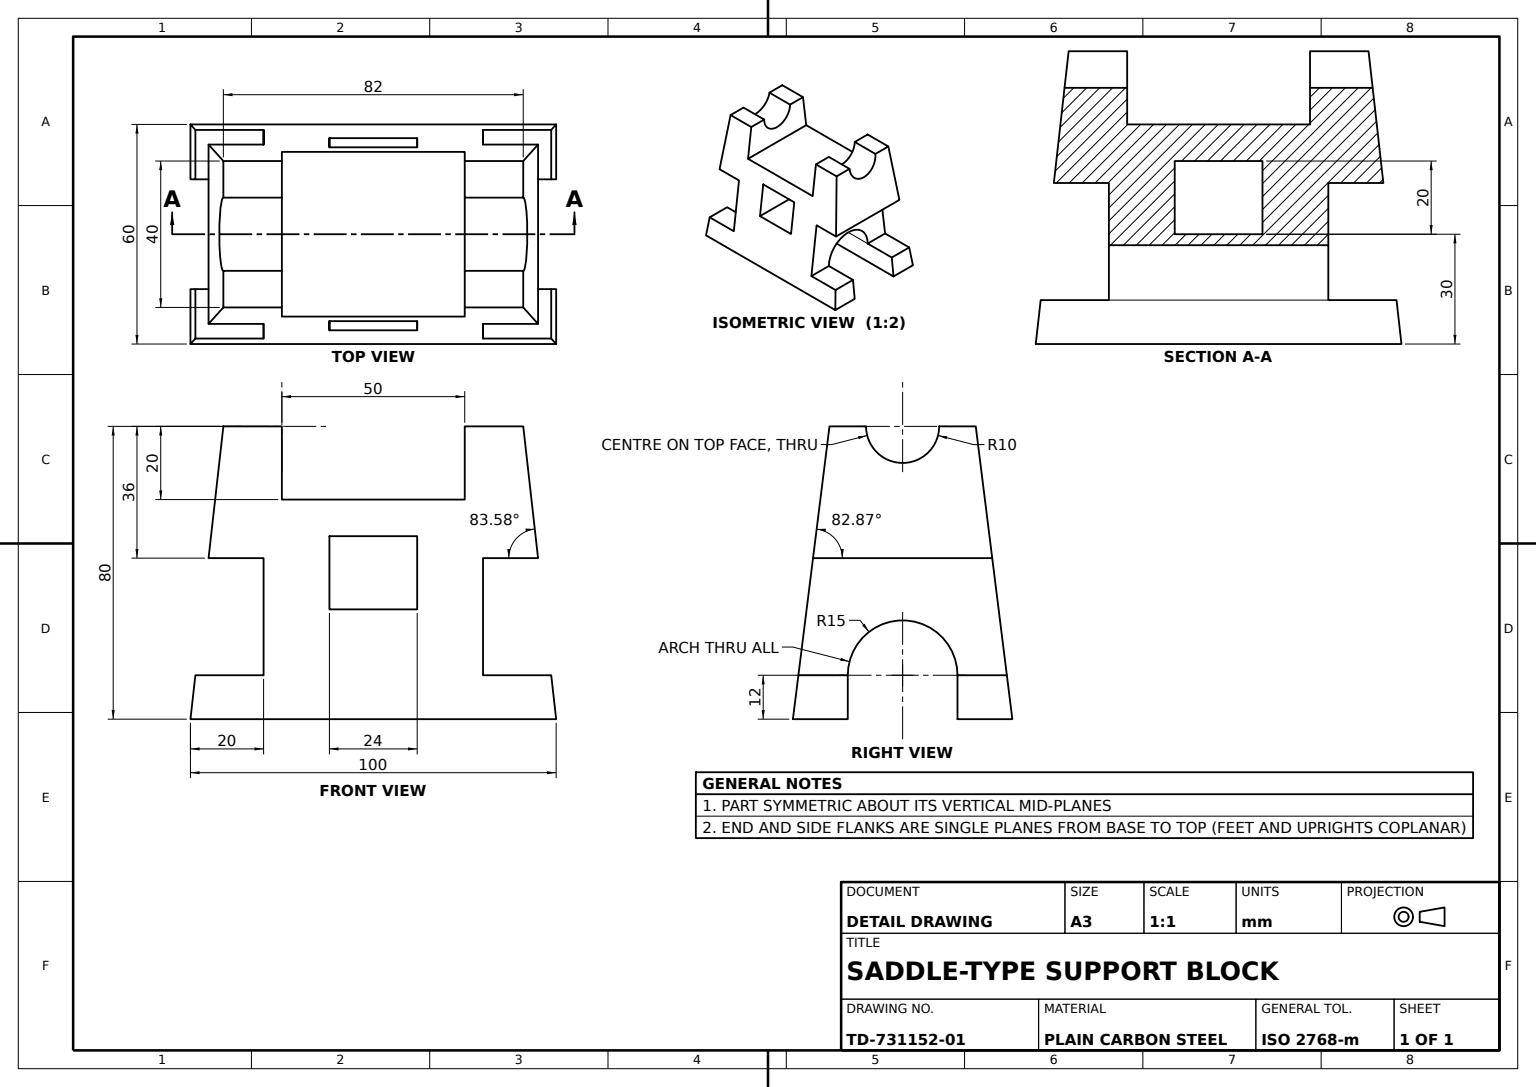
SolidWorks part; units mm, degrees
material "Plain Carbon Steel"
ref_plane "Front Plane" through (0, 0, 0) normal (0, 0, 1) x (1, 0, 0)
ref_plane "Top Plane" through (0, 0, 0) normal (0, 1, 0) x (1, 0, 0)
ref_plane "Right Plane" through (0, 0, 0) normal (1, 0, 0) x (0, 0, -1)
sketch "Base Profile Sketch" plane through (0, 0, 0) normal (0, 1, 0) x (1, 0, 0)
  line L1 (-50, -30) -> (50, -30)
  line L2 (-50, -30) -> (-50, 30)
  line L3 (-50, 30) -> (50, 30)
  line L4 (50, -30) -> (50, 30)
  line L5 (-50, -30) -> (50, 30) construction
  line L6 (-50, 30) -> (50, -30) construction
  point P0 (0, 0)
  dimension "D1" = 100
  dimension "D2" = 60
ref_plane "Top Profile Plane" through (0, 80, 0) normal (0, 1, 0) x (1, 0, 0)
sketch "Top Profile Sketch" plane through (0, 80, 0) normal (0, 1, 0) x (1, 0, 0)
  line L1 (-41, -20) -> (41, -20)
  line L2 (-41, -20) -> (-41, 20)
  line L3 (-41, 20) -> (41, 20)
  line L4 (41, -20) -> (41, 20)
  line L5 (-41, -20) -> (41, 20) construction
  line L6 (-41, 20) -> (41, -20) construction
  point P0 (0, 0)
  dimension "D1" = 82
  dimension "D2" = 40
loft "Tapered Block Loft" add profiles "Base Profile Sketch", "Top Profile Sketch"
sketch "Feet and Uprights Profile Sketch" plane through (0, 0, 0) normal (0, 0, 1) x (1, 0, 0)
  line L0 (-50, 0) -> (50, 0) construction
  line L1 (-30, 44) -> (-59.4094, 44)
  line L2 (-30, 44) -> (-30, 12)
  line L3 (-30, 12) -> (-59.4094, 12)
  line L4 (-59.4094, 44) -> (-59.4094, 12)
  line L5 (-41, 80) -> (41, 80) construction
  line L6 (0, 0) -> (0, 40.5816) construction
  line L7 (-25, 80) -> (25, 80)
  line L8 (-25, 80) -> (-25, 60)
  line L9 (-25, 60) -> (25, 60)
  line L10 (25, 80) -> (25, 60)
  line L11 (59.4094, 44) -> (59.4094, 12)
  line L12 (30, 12) -> (59.4094, 12)
  line L13 (30, 44) -> (30, 12)
  line L14 (30, 44) -> (59.4094, 44)
  point P19 (0, 60)
  dimension "D1" = 12
  dimension "D2" = 36
  dimension "D3" = 30
  dimension "D4" = 50
  dimension "D5" = 20
  dimension "D6" = 29.4094
extrude "Feet and Uprights Cut" cut sketch "Feet and Uprights Profile Sketch" against normal through all both and the other way through all
sketch "Base Arch Sketch" plane through (0, 0, 0) normal (1, 0, 0) x (0, 0, -1)
  line L0 (-20, 80) -> (20, 80) construction
  line L1 (-10, 80) -> (10, 80)
  arc A0 (-10, 80) -> (10, 80) centre (0, 80) ccw
  dimension "D1" = 10
  dimension "D2" = 20
extrude "Base Arch Cut" cut sketch "Base Arch Sketch" against normal through all both and the other way through all
sketch "Cradle Saddles Sketch" plane through (0, 0, 0) normal (1, 0, 0) x (0, 0, -1)
  line L0 (28.5, 12) -> (-28.5, 12) construction
  line L1 (-15, 12) -> (-15, 0)
  line L2 (-30, 0) -> (30, 0) construction
  line L3 (-15, 0) -> (15, 0)
  line L4 (15, 0) -> (15, 12)
  arc A0 (-15, 12) -> (15, 12) centre (0, 12) cw
  dimension "D1" = 15
extrude "Cradle Saddles Cut" cut sketch "Cradle Saddles Sketch" against normal through all both and the other way through all
sketch "Web Window Sketch" plane through (0, 0, 0) normal (0, 0, 1) x (1, 0, 0)
  line L0 (-50, 0) -> (50, 0) construction
  line L1 (-12, 30) -> (12, 30)
  line L2 (-12, 30) -> (-12, 50)
  line L3 (-12, 50) -> (12, 50)
  line L4 (12, 30) -> (12, 50)
  line L5 (-12, 30) -> (12, 50) construction
  line L6 (-12, 50) -> (12, 30) construction
  point P0 (0, 40)
  dimension "D1" = 24
  dimension "D2" = 20
  dimension "D3" = 30
extrude "Web Window Cut" cut sketch "Web Window Sketch" against normal through all both and the other way through all
